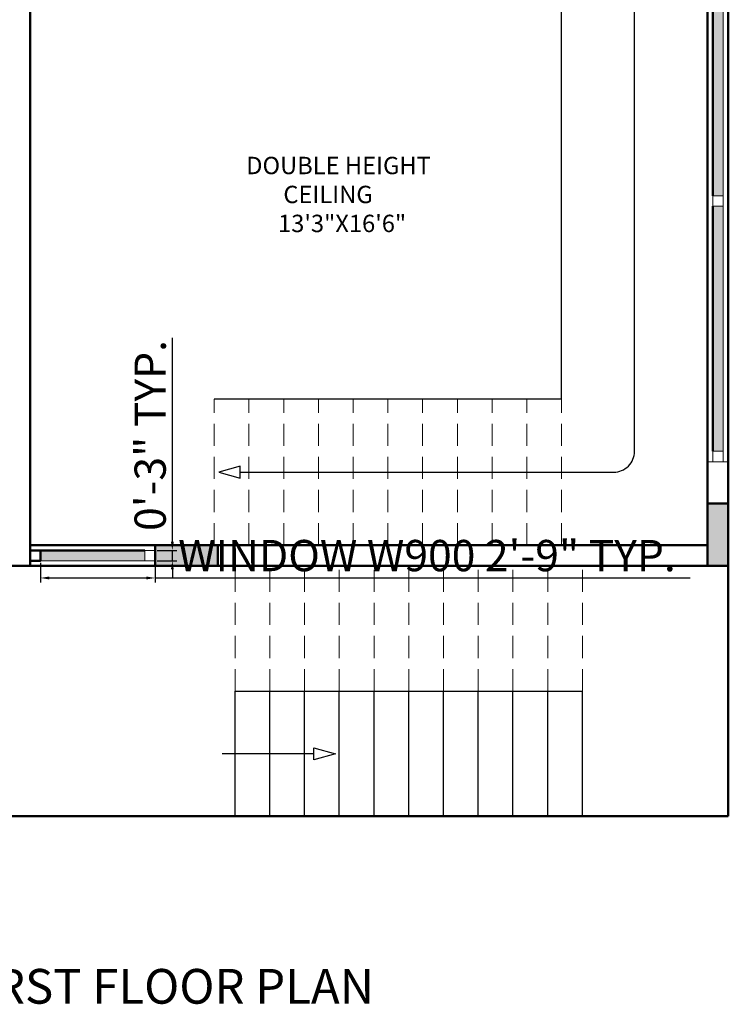
# Model space of a CAD drawing. Units: inches. Extents: x 3064 to 19385, y 846 to 15425.
# Tile 17 of 108: x 3785 to 3989, y 850 to 1134. Entities that reach past the tile are written whole.
import ezdxf

# ---------------------------------------------------------------- set-up
doc = ezdxf.new("R2010")
doc.units = ezdxf.units.IN
doc.linetypes.add('DASHED', pattern=[19.05, 12.7, -6.35])
for name, color, linetype, lineweight in [('A-ANNO-DIMS', 2, 'Continuous', 18), ('A-ANNO-TEXT', 7, 'Continuous', 25), ('A-AREA-IDEN', 3, 'Continuous', 18), ('A-COLS', 1, 'Continuous', 35), ('A-FLOR-STRS', 2, 'Continuous', 25), ('A-FLOR-STRS-OVHD', 2, 'DASHED', 18), ('A-GLAZ', 4, 'Continuous', 18), ('A-WALL', 7, 'Continuous', 50)]:
    doc.layers.add(name, color=color, linetype=linetype, lineweight=lineweight)
doc.styles.get("Standard").update_dxf_attribs({"font": 'arial.ttf'})
doc.dimstyles.new('ISO-25', dxfattribs={"dimtxt": 9, "dimasz": 2.5, "dimexe": 1.25, "dimexo": 0.625, "dimtad": 1, "dimdec": 1, "dimlunit": 3, "dimtxsty": 'Standard', "dimcen": 2.5, "dimadec": 0, "dimazin": 0, "dimtfac": 1, "dimtdec": 1, "dimtmove": 0, "dimatfit": 3, "dimfxl": 1, "dimarcsym": 0})

# ---------------------------------------------------------------- blocks, each defined once
blk = doc.blocks.new('WIN-1800-PAIR')
h = blk.add_hatch(color=256)
h.dxf.hatch_style = 1
h.paths.add_polyline_path([(0, 0), (3, 0), (3, 70.5), (0, 70.5)])
h.paths.add_polyline_path([(3, 144), (0, 144), (0, 73.5), (3, 73.5)])
blk.add_line((3, 144), (3, 73.5))
blk.add_lwpolyline([(3, 144), (0, 144), (0, 147), (3, 147)], close=True)
blk = doc.blocks.new('WIN-900')
blk.add_line((0, 0), (30, 0))
blk.add_lwpolyline([(30, 0), (30, 3), (33, 3), (33, 0)], close=True)
blk = doc.blocks.new('WIN-2000')
blk.add_line((3, 0), (3, 70.5))
blk.add_lwpolyline([(3, 70.5), (0, 70.5), (0, 73.5), (3, 73.5)], close=True)
blk = doc.blocks.new('*D435')
at = {"layer": 'A-ANNO-DIMS', "color": 0, "lineweight": -2, "transparency": 16777216}
for p, q in [((3791.36, 977.21), (3791.36, 971.64)), ((3824.36, 977.21), (3824.36, 971.64)), ((3793.86, 972.89), (3821.86, 972.89)), ((3824.36, 972.89), (3978.33, 972.89))]:
    blk.add_line(p, q, dxfattribs=at)
at = {"layer": 'A-ANNO-DIMS', "color": 0, "transparency": 16777216}
for points in [[(3793.86, 973.31), (3793.86, 972.47), (3791.36, 972.89)], [(3821.86, 973.31), (3821.86, 972.47), (3824.36, 972.89)]]:
    blk.add_solid(points, dxfattribs=at)
at = {"layer": 'Defpoints', "color": 0, "transparency": 16777216}
for p in [(3791.36, 977.84), (3824.36, 977.84), (3824.36, 972.89)]:
    blk.add_point(p, dxfattribs=at)
at = {"layer": 'A-ANNO-DIMS', "color": 0, "transparency": 16777216, "insert": (3902.6, 978.17), "char_height": 9, "attachment_point": 5}
blk.add_mtext('WINDOW W900 2\'-9" TYP.', dxfattribs=at)
blk = doc.blocks.new('*D436')
at = {"layer": 'A-ANNO-DIMS', "color": 0, "lineweight": -2, "transparency": 16777216}
for p, q in [((3829.31, 983.34), (3829.31, 1041.95)), ((3824.98, 980.84), (3830.56, 980.84)), ((3829.31, 977.84), (3829.31, 980.84)), ((3824.98, 977.84), (3830.56, 977.84)), ((3829.31, 975.34), (3829.31, 972.84))]:
    blk.add_line(p, q, dxfattribs=at)
at = {"layer": 'A-ANNO-DIMS', "color": 0, "transparency": 16777216}
for points in [[(3828.89, 983.34), (3829.73, 983.34), (3829.31, 980.84)], [(3828.89, 975.34), (3829.73, 975.34), (3829.31, 977.84)]]:
    blk.add_solid(points, dxfattribs=at)
at = {"layer": 'Defpoints', "color": 0, "transparency": 16777216}
for p in [(3824.36, 980.84), (3829.31, 980.84), (3824.36, 977.84)]:
    blk.add_point(p, dxfattribs=at)
at = {"layer": 'A-ANNO-DIMS', "color": 0, "transparency": 16777216, "insert": (3824.09, 1013.89), "char_height": 9, "attachment_point": 5, "rotation": 90}
blk.add_mtext('0\'-3" TYP.', dxfattribs=at)

msp = doc.modelspace()

# ---------------------------------------------------------------- hatches: boundary and pattern name
at = {"layer": 'A-COLS'}
h = msp.add_hatch(color=256, dxfattribs=at)
h.dxf.hatch_style = 1
h.paths.add_polyline_path([(3983.36, 976.34), (3989.36, 976.34), (3989.36, 994.34), (3983.36, 994.34)])
h = msp.add_hatch(color=256, dxfattribs=at)
h.dxf.hatch_style = 1
h.paths.add_polyline_path([(3842.36, 976.34), (3842.36, 982.34), (3824.36, 982.34), (3824.36, 976.34)])
at = {"layer": 'A-GLAZ'}
h = msp.add_hatch(color=256, dxfattribs=at)
h.dxf.hatch_style = 1
h.paths.add_polyline_path([(3791.36, 980.84), (3791.36, 977.84), (3821.36, 977.84), (3821.36, 980.84)])

# ---------------------------------------------------------------- linework, layer by layer
at = {"layer": 'A-FLOR-STRS'}
for p, q in [((3941.36, 1024.34), (3941.36, 1180.34)), ((3941.36, 1024.34), (3841.36, 1024.34)), ((3847.36, 904.34), (3847.36, 940.34)), ((3847.36, 940.34), (3947.36, 940.34)), ((3857.36, 904.34), (3857.36, 940.34)), ((3867.36, 904.34), (3867.36, 940.34)), ((3877.36, 904.34), (3877.36, 940.34)), ((3887.36, 904.34), (3887.36, 940.34)), ((3897.36, 904.34), (3897.36, 940.34)), ((3907.36, 904.34), (3907.36, 940.34)), ((3917.36, 904.34), (3917.36, 940.34)), ((3927.36, 904.34), (3927.36, 940.34)), ((3937.36, 904.34), (3937.36, 940.34)), ((3947.36, 904.34), (3947.36, 940.34)), ((3870.06, 922.34), (3843.67, 922.34))]:
    msp.add_line(p, q, dxfattribs=at)
msp.add_lwpolyline([(3848.85, 1003.34), (3956.36, 1003.34, 0.414214), (3962.36, 1009.34), (3962.36, 1153.34, 0.414214), (3956.36, 1159.34), (3829.36, 1159.34)], format="xyb", dxfattribs=at)
for points in [[(3842.65, 1003.34), (3848.85, 1001.61), (3848.85, 1005.07)], [(3876.26, 922.34), (3870.06, 920.61), (3870.06, 924.07)]]:
    msp.add_lwpolyline(points, close=True, dxfattribs=at)
at = {"layer": 'A-FLOR-STRS-OVHD', "ltscale": 0.5}
for p, q in [((3841.36, 982.34), (3841.36, 1024.34)), ((3851.36, 982.34), (3851.36, 1024.34)), ((3861.36, 982.34), (3861.36, 1024.34)), ((3871.36, 982.34), (3871.36, 1024.34)), ((3881.36, 982.34), (3881.36, 1024.34)), ((3891.36, 982.34), (3891.36, 1024.34)), ((3901.36, 982.34), (3901.36, 1024.34)), ((3911.36, 982.34), (3911.36, 1024.34)), ((3921.36, 982.34), (3921.36, 1024.34)), ((3931.36, 982.34), (3931.36, 1024.34)), ((3941.36, 982.34), (3941.36, 1024.34)), ((3847.36, 940.34), (3847.36, 976.34)), ((3857.36, 940.34), (3857.36, 976.34)), ((3867.36, 940.34), (3867.36, 976.34)), ((3877.36, 940.34), (3877.36, 976.34)), ((3887.36, 940.34), (3887.36, 976.34)), ((3897.36, 940.34), (3897.36, 976.34)), ((3907.36, 940.34), (3907.36, 976.34)), ((3917.36, 940.34), (3917.36, 976.34)), ((3927.36, 940.34), (3927.36, 976.34)), ((3937.36, 940.34), (3937.36, 976.34)), ((3947.36, 940.34), (3947.36, 976.34))]:
    msp.add_line(p, q, dxfattribs=at)
at = {"layer": 'A-GLAZ'}
msp.add_line((3989.36, 1006.34), (3983.36, 1006.34), dxfattribs=at)
msp.add_line((3989.36, 1006.34), (3983.36, 1006.34), dxfattribs=at)
msp.add_lwpolyline([(3987.86, 1006.34), (3984.86, 1006.34), (3984.86, 1009.34), (3987.86, 1009.34)], close=True, dxfattribs=at)
at = {"layer": 'A-WALL'}
for p, q in [((3989.36, 904.34), (3989.36, 1396.34)), ((3983.36, 982.34), (3983.36, 1180.34)), ((3984.86, 1153.34), (3984.86, 1082.84)), ((3788.36, 1144.34), (3788.36, 976.34)), ((3984.86, 1009.34), (3984.86, 1079.84)), ((3983.36, 982.34), (3788.36, 982.34)), ((3788.36, 976.34), (3788.36, 982.34)), ((3791.36, 980.84), (3821.36, 980.84)), ((3824.36, 976.34), (3824.36, 982.34)), ((3824.36, 976.34), (3824.36, 982.34)), ((3989.36, 976.34), (3647.36, 976.34)), ((3647.36, 904.34), (3989.36, 904.34))]:
    msp.add_line(p, q, dxfattribs=at)
for points in [[(3989.36, 976.34), (3989.36, 994.34), (3983.36, 994.34), (3983.36, 976.34)], [(3788.36, 977.84), (3788.36, 980.84), (3791.36, 980.84), (3791.36, 977.84)], [(3842.36, 982.34), (3824.36, 982.34), (3824.36, 976.34), (3842.36, 976.34)]]:
    msp.add_lwpolyline(points, close=True, dxfattribs=at)

# ---------------------------------------------------------------- block references
at = {"layer": 'A-GLAZ'}
for name, p in [('WIN-1800-PAIR', (3984.86, 1009.34)), ('WIN-2000', (3984.86, 1009.34)), ('WIN-900', (3791.36, 977.84))]:
    msp.add_blockref(name, p, dxfattribs=at)

# ---------------------------------------------------------------- texts
at = {"layer": 'A-ANNO-TEXT', "insert": (3766.7, 860.41), "char_height": 10, "attachment_point": 1}
msp.add_mtext_dynamic_manual_height_columns('FIRST FLOOR PLAN', width=200.9739, gutter_width=12.5, heights=[0], dxfattribs=at)
at = {"layer": 'A-AREA-IDEN', "insert": (3850.57, 1094.07), "char_height": 5, "attachment_point": 1}
msp.add_mtext_dynamic_manual_height_columns('DOUBLE HEIGHT \\P       CEILING            \\P      13\'3"X16\'6"', width=57.0817, gutter_width=12.5, heights=[0], dxfattribs=at)

# ---------------------------------------------------------------- dimensions: what is measured, and where the dimension line sits
at = {"layer": 'A-ANNO-DIMS'}
dim = msp.add_linear_dim(base=(3829.31, 980.84), p1=(3824.36, 977.84), p2=(3824.36, 980.84), angle=90, text='<> TYP.', dimstyle='ISO-25', override={"dimdec": 1, "dimrnd": 0, "dimzin": 1, "dimlunit": 4, "dimfrac": 2}, dxfattribs=at)
dim.commit()
dim.dimension.update_dxf_attribs({"geometry": '*D436', "text_midpoint": (3824.09, 1013.89)})
dim = msp.add_linear_dim(base=(3824.36, 972.89), p1=(3791.36, 977.84), p2=(3824.36, 977.84), text='WINDOW W900 <> TYP.', dimstyle='ISO-25', override={"dimdec": 1, "dimrnd": 0, "dimzin": 1, "dimlunit": 4, "dimfrac": 2}, dxfattribs=at)
dim.commit()
dim.dimension.update_dxf_attribs({"geometry": '*D435', "text_midpoint": (3902.6, 978.17)})

doc.saveas('drawing.dxf')
